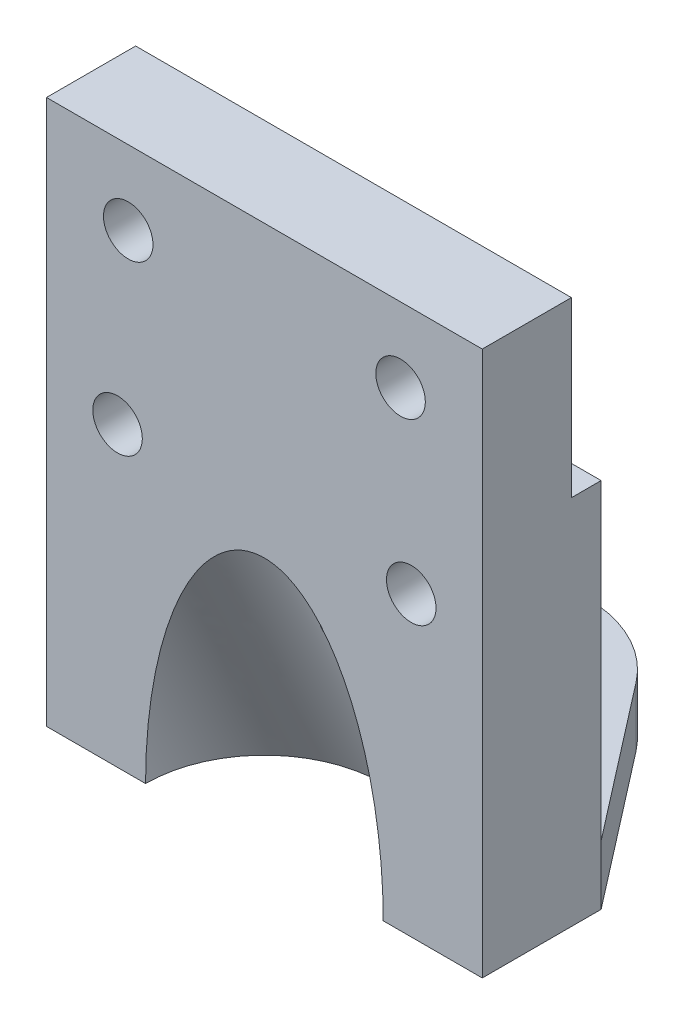
ISO-10303-21;
HEADER;
FILE_DESCRIPTION(('STEP AP214'),'2;1');
FILE_NAME('part.step','',(''),(''),'','','');
FILE_SCHEMA(('AUTOMOTIVE_DESIGN { 1 0 10303 214 1 1 1 1 }'));
ENDSEC;
DATA;
#1=APPLICATION_CONTEXT('core data for automotive mechanical design processes');
#2=APPLICATION_PROTOCOL_DEFINITION('international standard','automotive_design',2000,#1);
#3=PRODUCT_CONTEXT('',#1,'mechanical');
#4=PRODUCT('Part','Part','',(#3));
#5=PRODUCT_RELATED_PRODUCT_CATEGORY('part','',(#4));
#6=PRODUCT_DEFINITION_FORMATION('','',#4);
#7=PRODUCT_DEFINITION_CONTEXT('part definition',#1,'design');
#8=PRODUCT_DEFINITION('design','',#6,#7);
#9=PRODUCT_DEFINITION_SHAPE('','',#8);
#10=(LENGTH_UNIT() NAMED_UNIT(*) SI_UNIT(.MILLI.,.METRE.));
#11=(NAMED_UNIT(*) PLANE_ANGLE_UNIT() SI_UNIT($,.RADIAN.));
#12=(NAMED_UNIT(*) SI_UNIT($,.STERADIAN.) SOLID_ANGLE_UNIT());
#13=UNCERTAINTY_MEASURE_WITH_UNIT(LENGTH_MEASURE(1.E-05),#10,'distance_accuracy_value','');
#14=(GEOMETRIC_REPRESENTATION_CONTEXT(3) GLOBAL_UNCERTAINTY_ASSIGNED_CONTEXT((#13)) GLOBAL_UNIT_ASSIGNED_CONTEXT((#10,
#11,#12)) REPRESENTATION_CONTEXT('',''));
#15=CARTESIAN_POINT('',(0.,0.,0.));
#16=DIRECTION('',(0.,0.,1.));
#17=DIRECTION('',(1.,0.,0.));
#18=AXIS2_PLACEMENT_3D('',#15,#16,#17);
#19=CARTESIAN_POINT('',(-44.,75.,-24.));
#20=DIRECTION('',(0.,0.,1.));
#21=DIRECTION('',(1.,0.,0.));
#22=AXIS2_PLACEMENT_3D('',#19,#20,#21);
#23=PLANE('',#22);
#24=CARTESIAN_POINT('',(-29.6529204550313,60.,-24.));
#25=DIRECTION('',(0.,0.,1.));
#26=DIRECTION('',(1.,0.,0.));
#27=AXIS2_PLACEMENT_3D('',#24,#25,#26);
#28=CIRCLE('',#27,5.);
#29=CARTESIAN_POINT('',(-24.6529204550313,60.,-24.));
#30=VERTEX_POINT('',#29);
#31=EDGE_CURVE('E140',#30,#30,#28,.F.);
#32=ORIENTED_EDGE('',*,*,#31,.F.);
#33=EDGE_LOOP('',(#32));
#34=FACE_BOUND('',#33,.T.);
#35=CARTESIAN_POINT('',(29.6529204550313,60.,-24.));
#36=DIRECTION('',(0.,0.,1.));
#37=DIRECTION('',(1.,0.,0.));
#38=AXIS2_PLACEMENT_3D('',#35,#36,#37);
#39=CIRCLE('',#38,5.);
#40=CARTESIAN_POINT('',(34.6529204550313,60.,-24.));
#41=VERTEX_POINT('',#40);
#42=EDGE_CURVE('E257',#41,#41,#39,.F.);
#43=ORIENTED_EDGE('',*,*,#42,.F.);
#44=EDGE_LOOP('',(#43));
#45=FACE_BOUND('',#44,.T.);
#46=DIRECTION('',(1.,0.,0.));
#47=VECTOR('',#46,1.);
#48=CARTESIAN_POINT('',(0.,12.,-24.));
#49=LINE('',#48,#47);
#50=CARTESIAN_POINT('',(-44.,12.,-24.));
#51=VERTEX_POINT('',#50);
#52=CARTESIAN_POINT('',(44.,12.,-24.));
#53=VERTEX_POINT('',#52);
#54=EDGE_CURVE('E75',#51,#53,#49,.T.);
#55=ORIENTED_EDGE('',*,*,#54,.F.);
#56=DIRECTION('',(0.,-1.,0.));
#57=VECTOR('',#56,1.);
#58=CARTESIAN_POINT('',(-44.,75.,-24.));
#59=LINE('',#58,#57);
#60=CARTESIAN_POINT('',(-44.,75.,-24.));
#61=VERTEX_POINT('',#60);
#62=EDGE_CURVE('E221',#61,#51,#59,.T.);
#63=ORIENTED_EDGE('',*,*,#62,.F.);
#64=DIRECTION('',(-1.,0.,0.));
#65=VECTOR('',#64,1.);
#66=CARTESIAN_POINT('',(-44.,75.,-24.));
#67=LINE('',#66,#65);
#68=CARTESIAN_POINT('',(44.,75.,-24.));
#69=VERTEX_POINT('',#68);
#70=EDGE_CURVE('E211',#69,#61,#67,.T.);
#71=ORIENTED_EDGE('',*,*,#70,.F.);
#72=DIRECTION('',(0.,-1.,0.));
#73=VECTOR('',#72,1.);
#74=CARTESIAN_POINT('',(44.,75.,-24.));
#75=LINE('',#74,#73);
#76=EDGE_CURVE('E172',#69,#53,#75,.T.);
#77=ORIENTED_EDGE('',*,*,#76,.T.);
#78=EDGE_LOOP('',(#55,#63,#71,#77));
#79=FACE_BOUND('',#78,.T.);
#80=ADVANCED_FACE('F44',(#34,#45,#79),#23,.F.);
#81=CARTESIAN_POINT('',(0.,0.,-18.));
#82=DIRECTION('',(0.,0.,1.));
#83=DIRECTION('',(1.,0.,0.));
#84=AXIS2_PLACEMENT_3D('',#81,#82,#83);
#85=PLANE('',#84);
#86=CARTESIAN_POINT('',(27.5,95.,-18.));
#87=DIRECTION('',(0.,0.,1.));
#88=DIRECTION('',(1.,0.,0.));
#89=AXIS2_PLACEMENT_3D('',#86,#87,#88);
#90=CIRCLE('',#89,5.);
#91=CARTESIAN_POINT('',(32.5,95.,-18.));
#92=VERTEX_POINT('',#91);
#93=EDGE_CURVE('E199',#92,#92,#90,.T.);
#94=ORIENTED_EDGE('',*,*,#93,.T.);
#95=EDGE_LOOP('',(#94));
#96=FACE_BOUND('',#95,.T.);
#97=CARTESIAN_POINT('',(-27.5,95.,-18.));
#98=DIRECTION('',(0.,0.,1.));
#99=DIRECTION('',(1.,0.,0.));
#100=AXIS2_PLACEMENT_3D('',#97,#98,#99);
#101=CIRCLE('',#100,5.);
#102=CARTESIAN_POINT('',(-22.5,95.,-18.));
#103=VERTEX_POINT('',#102);
#104=EDGE_CURVE('E246',#103,#103,#101,.T.);
#105=ORIENTED_EDGE('',*,*,#104,.T.);
#106=EDGE_LOOP('',(#105));
#107=FACE_BOUND('',#106,.T.);
#108=DIRECTION('',(1.,0.,0.));
#109=VECTOR('',#108,1.);
#110=CARTESIAN_POINT('',(-44.,75.,-18.));
#111=LINE('',#110,#109);
#112=CARTESIAN_POINT('',(-44.,75.,-18.));
#113=VERTEX_POINT('',#112);
#114=CARTESIAN_POINT('',(44.,75.,-18.));
#115=VERTEX_POINT('',#114);
#116=EDGE_CURVE('E220',#113,#115,#111,.T.);
#117=ORIENTED_EDGE('',*,*,#116,.F.);
#118=DIRECTION('',(0.,-1.,0.));
#119=VECTOR('',#118,1.);
#120=CARTESIAN_POINT('',(-44.,110.,-18.));
#121=LINE('',#120,#119);
#122=CARTESIAN_POINT('',(-44.,110.,-18.));
#123=VERTEX_POINT('',#122);
#124=EDGE_CURVE('E160',#123,#113,#121,.T.);
#125=ORIENTED_EDGE('',*,*,#124,.F.);
#126=DIRECTION('',(-1.,0.,0.));
#127=VECTOR('',#126,1.);
#128=CARTESIAN_POINT('',(-44.,110.,-18.));
#129=LINE('',#128,#127);
#130=CARTESIAN_POINT('',(44.,110.,-18.));
#131=VERTEX_POINT('',#130);
#132=EDGE_CURVE('E150',#131,#123,#129,.T.);
#133=ORIENTED_EDGE('',*,*,#132,.F.);
#134=DIRECTION('',(0.,1.,0.));
#135=VECTOR('',#134,1.);
#136=CARTESIAN_POINT('',(44.,110.,-18.));
#137=LINE('',#136,#135);
#138=EDGE_CURVE('E143',#115,#131,#137,.T.);
#139=ORIENTED_EDGE('',*,*,#138,.F.);
#140=EDGE_LOOP('',(#117,#125,#133,#139));
#141=FACE_BOUND('',#140,.T.);
#142=ADVANCED_FACE('F310',(#96,#107,#141),#85,.F.);
#143=CARTESIAN_POINT('',(44.,110.,-18.));
#144=DIRECTION('',(1.,0.,0.));
#145=DIRECTION('',(0.,1.,0.));
#146=AXIS2_PLACEMENT_3D('',#143,#144,#145);
#147=PLANE('',#146);
#148=DIRECTION('',(0.,1.,0.));
#149=VECTOR('',#148,1.);
#150=CARTESIAN_POINT('',(44.,110.,0.));
#151=LINE('',#150,#149);
#152=CARTESIAN_POINT('',(44.,0.,0.));
#153=VERTEX_POINT('',#152);
#154=CARTESIAN_POINT('',(44.,110.,0.));
#155=VERTEX_POINT('',#154);
#156=EDGE_CURVE('E171',#153,#155,#151,.T.);
#157=ORIENTED_EDGE('',*,*,#156,.F.);
#158=DIRECTION('',(0.,0.,1.));
#159=VECTOR('',#158,1.);
#160=CARTESIAN_POINT('',(44.,0.,-18.));
#161=LINE('',#160,#159);
#162=CARTESIAN_POINT('',(44.,0.,-24.));
#163=VERTEX_POINT('',#162);
#164=EDGE_CURVE('E56',#163,#153,#161,.T.);
#165=ORIENTED_EDGE('',*,*,#164,.F.);
#166=DIRECTION('',(0.,-1.,0.));
#167=VECTOR('',#166,1.);
#168=CARTESIAN_POINT('',(44.,12.,-24.));
#169=LINE('',#168,#167);
#170=EDGE_CURVE('E207',#53,#163,#169,.T.);
#171=ORIENTED_EDGE('',*,*,#170,.F.);
#172=ORIENTED_EDGE('',*,*,#76,.F.);
#173=DIRECTION('',(0.,0.,-1.));
#174=VECTOR('',#173,1.);
#175=CARTESIAN_POINT('',(44.,75.,-24.));
#176=LINE('',#175,#174);
#177=EDGE_CURVE('E204',#115,#69,#176,.T.);
#178=ORIENTED_EDGE('',*,*,#177,.F.);
#179=ORIENTED_EDGE('',*,*,#138,.T.);
#180=DIRECTION('',(0.,0.,1.));
#181=VECTOR('',#180,1.);
#182=CARTESIAN_POINT('',(44.,110.,-18.));
#183=LINE('',#182,#181);
#184=EDGE_CURVE('E156',#131,#155,#183,.T.);
#185=ORIENTED_EDGE('',*,*,#184,.T.);
#186=EDGE_LOOP('',(#157,#165,#171,#172,#178,#179,#185));
#187=FACE_BOUND('',#186,.T.);
#188=ADVANCED_FACE('F50',(#187),#147,.T.);
#189=CARTESIAN_POINT('',(-44.,0.,-18.));
#190=DIRECTION('',(0.,-1.,0.));
#191=DIRECTION('',(0.,0.,-1.));
#192=AXIS2_PLACEMENT_3D('',#189,#190,#191);
#193=PLANE('',#192);
#194=CARTESIAN_POINT('',(0.,0.,0.));
#195=DIRECTION('',(0.,-1.,0.));
#196=DIRECTION('',(0.,0.,-1.));
#197=AXIS2_PLACEMENT_3D('',#194,#195,#196);
#198=CIRCLE('',#197,24.);
#199=CARTESIAN_POINT('',(-24.,0.,0.));
#200=VERTEX_POINT('',#199);
#201=CARTESIAN_POINT('',(24.,0.,0.));
#202=VERTEX_POINT('',#201);
#203=EDGE_CURVE('E61',#200,#202,#198,.T.);
#204=ORIENTED_EDGE('',*,*,#203,.F.);
#205=DIRECTION('',(1.,0.,0.));
#206=VECTOR('',#205,1.);
#207=CARTESIAN_POINT('',(-44.,0.,0.));
#208=LINE('',#207,#206);
#209=CARTESIAN_POINT('',(-44.,0.,0.));
#210=VERTEX_POINT('',#209);
#211=EDGE_CURVE('E131',#210,#200,#208,.T.);
#212=ORIENTED_EDGE('',*,*,#211,.F.);
#213=DIRECTION('',(0.,0.,1.));
#214=VECTOR('',#213,1.);
#215=CARTESIAN_POINT('',(-44.,0.,-18.));
#216=LINE('',#215,#214);
#217=CARTESIAN_POINT('',(-44.,0.,-24.));
#218=VERTEX_POINT('',#217);
#219=EDGE_CURVE('E155',#218,#210,#216,.T.);
#220=ORIENTED_EDGE('',*,*,#219,.F.);
#221=DIRECTION('',(0.612114706356877,0.,-0.790768984129773));
#222=VECTOR('',#221,1.);
#223=CARTESIAN_POINT('',(-39.1308775839132,0.,-30.2902442084566));
#224=LINE('',#223,#222);
#225=CARTESIAN_POINT('',(-19.7692246032443,0.,-55.3028676589219));
#226=VERTEX_POINT('',#225);
#227=EDGE_CURVE('E183',#218,#226,#224,.T.);
#228=ORIENTED_EDGE('',*,*,#227,.T.);
#229=CARTESIAN_POINT('',(0.,0.,-40.));
#230=DIRECTION('',(0.,-1.,0.));
#231=DIRECTION('',(0.,0.,-1.));
#232=AXIS2_PLACEMENT_3D('',#229,#230,#231);
#233=CIRCLE('',#232,25.);
#234=CARTESIAN_POINT('',(19.7692246032443,0.,-55.3028676589219));
#235=VERTEX_POINT('',#234);
#236=EDGE_CURVE('E192',#226,#235,#233,.T.);
#237=ORIENTED_EDGE('',*,*,#236,.T.);
#238=DIRECTION('',(0.612114706356877,0.,0.790768984129774));
#239=VECTOR('',#238,1.);
#240=CARTESIAN_POINT('',(39.1308775839132,0.,-30.2902442084566));
#241=LINE('',#240,#239);
#242=EDGE_CURVE('E191',#235,#163,#241,.T.);
#243=ORIENTED_EDGE('',*,*,#242,.T.);
#244=ORIENTED_EDGE('',*,*,#164,.T.);
#245=EDGE_CURVE('E136',#202,#153,#208,.T.);
#246=ORIENTED_EDGE('',*,*,#245,.F.);
#247=EDGE_LOOP('',(#204,#212,#220,#228,#237,#243,#244,#246));
#248=FACE_BOUND('',#247,.T.);
#249=CARTESIAN_POINT('',(0.,0.,-40.));
#250=DIRECTION('',(0.,-1.,0.));
#251=DIRECTION('',(0.,0.,-1.));
#252=AXIS2_PLACEMENT_3D('',#249,#250,#251);
#253=CIRCLE('',#252,9.5);
#254=CARTESIAN_POINT('',(0.,0.,-49.5));
#255=VERTEX_POINT('',#254);
#256=EDGE_CURVE('E195',#255,#255,#253,.T.);
#257=ORIENTED_EDGE('',*,*,#256,.F.);
#258=EDGE_LOOP('',(#257));
#259=FACE_BOUND('',#258,.T.);
#260=ADVANCED_FACE('F132',(#248,#259),#193,.T.);
#261=CARTESIAN_POINT('',(-44.,110.,-18.));
#262=DIRECTION('',(-1.,0.,0.));
#263=DIRECTION('',(0.,-1.,0.));
#264=AXIS2_PLACEMENT_3D('',#261,#262,#263);
#265=PLANE('',#264);
#266=DIRECTION('',(0.,-1.,0.));
#267=VECTOR('',#266,1.);
#268=CARTESIAN_POINT('',(-44.,110.,0.));
#269=LINE('',#268,#267);
#270=CARTESIAN_POINT('',(-44.,110.,0.));
#271=VERTEX_POINT('',#270);
#272=EDGE_CURVE('E144',#271,#210,#269,.T.);
#273=ORIENTED_EDGE('',*,*,#272,.F.);
#274=DIRECTION('',(0.,0.,1.));
#275=VECTOR('',#274,1.);
#276=CARTESIAN_POINT('',(-44.,110.,-18.));
#277=LINE('',#276,#275);
#278=EDGE_CURVE('E153',#123,#271,#277,.T.);
#279=ORIENTED_EDGE('',*,*,#278,.F.);
#280=ORIENTED_EDGE('',*,*,#124,.T.);
#281=DIRECTION('',(0.,0.,1.));
#282=VECTOR('',#281,1.);
#283=CARTESIAN_POINT('',(-44.,75.,-24.));
#284=LINE('',#283,#282);
#285=EDGE_CURVE('E217',#61,#113,#284,.T.);
#286=ORIENTED_EDGE('',*,*,#285,.F.);
#287=ORIENTED_EDGE('',*,*,#62,.T.);
#288=DIRECTION('',(0.,-1.,0.));
#289=VECTOR('',#288,1.);
#290=CARTESIAN_POINT('',(-44.,12.,-24.));
#291=LINE('',#290,#289);
#292=EDGE_CURVE('E179',#51,#218,#291,.T.);
#293=ORIENTED_EDGE('',*,*,#292,.T.);
#294=ORIENTED_EDGE('',*,*,#219,.T.);
#295=EDGE_LOOP('',(#273,#279,#280,#286,#287,#293,#294));
#296=FACE_BOUND('',#295,.T.);
#297=ADVANCED_FACE('F178',(#296),#265,.T.);
#298=CARTESIAN_POINT('',(-44.,110.,-18.));
#299=DIRECTION('',(0.,1.,0.));
#300=DIRECTION('',(0.,0.,1.));
#301=AXIS2_PLACEMENT_3D('',#298,#299,#300);
#302=PLANE('',#301);
#303=DIRECTION('',(-1.,0.,0.));
#304=VECTOR('',#303,1.);
#305=CARTESIAN_POINT('',(-44.,110.,0.));
#306=LINE('',#305,#304);
#307=EDGE_CURVE('E173',#155,#271,#306,.T.);
#308=ORIENTED_EDGE('',*,*,#307,.F.);
#309=ORIENTED_EDGE('',*,*,#184,.F.);
#310=ORIENTED_EDGE('',*,*,#132,.T.);
#311=ORIENTED_EDGE('',*,*,#278,.T.);
#312=EDGE_LOOP('',(#308,#309,#310,#311));
#313=FACE_BOUND('',#312,.T.);
#314=ADVANCED_FACE('F176',(#313),#302,.T.);
#315=CARTESIAN_POINT('',(0.,0.,0.));
#316=DIRECTION('',(0.,0.,1.));
#317=DIRECTION('',(1.,0.,0.));
#318=AXIS2_PLACEMENT_3D('',#315,#316,#317);
#319=PLANE('',#318);
#320=CARTESIAN_POINT('',(24.,0.,0.));
#321=CARTESIAN_POINT('',(23.9999836526665,0.822487909594253,0.));
#322=CARTESIAN_POINT('',(23.9908057653102,1.64497853466898,0.));
#323=CARTESIAN_POINT('',(23.9540097607918,3.28956132881042,0.));
#324=CARTESIAN_POINT('',(23.926391316428,4.11165349054796,0.));
#325=CARTESIAN_POINT('',(23.8525962581262,5.75502367391495,0.));
#326=CARTESIAN_POINT('',(23.8064192507315,6.57630167791351,0.));
#327=CARTESIAN_POINT('',(23.6952719286014,8.21758441968101,0.));
#328=CARTESIAN_POINT('',(23.6303016801107,9.03758916192785,0.));
#329=CARTESIAN_POINT('',(23.4812324663408,10.6759416559738,0.));
#330=CARTESIAN_POINT('',(23.3971316451274,11.4942892392287,0.));
#331=CARTESIAN_POINT('',(23.2093684539698,13.1287360620571,0.));
#332=CARTESIAN_POINT('',(23.1057062152105,13.9448353166713,0.));
#333=CARTESIAN_POINT('',(22.8782379124427,15.5744315564589,0.));
#334=CARTESIAN_POINT('',(22.7544269129195,16.3879278541186,0.));
#335=CARTESIAN_POINT('',(22.4859934425246,18.011484999328,0.));
#336=CARTESIAN_POINT('',(22.3413710215974,18.8215458551175,0.));
#337=CARTESIAN_POINT('',(22.0303366920778,20.4382530974152,0.));
#338=CARTESIAN_POINT('',(21.8639049278322,21.2448956725252,0.));
#339=CARTESIAN_POINT('',(21.5083419460309,22.8531858262733,0.));
#340=CARTESIAN_POINT('',(21.3192104530091,23.6548333441712,0.));
#341=CARTESIAN_POINT('',(20.9171806973682,25.2515514932186,0.));
#342=CARTESIAN_POINT('',(20.7042994691011,26.0466264044593,0.));
#343=CARTESIAN_POINT('',(20.2532181884177,27.6295613335899,0.));
#344=CARTESIAN_POINT('',(20.0150191240817,28.4174216317423,0.));
#345=CARTESIAN_POINT('',(19.5811011965835,29.7680075743554,0.));
#346=CARTESIAN_POINT('',(19.3918229003344,30.3328070716185,0.));
#347=CARTESIAN_POINT('',(18.9983197094544,31.4571678498858,0.));
#348=CARTESIAN_POINT('',(18.7940953229582,32.0167293082431,0.));
#349=CARTESIAN_POINT('',(18.3694400982678,33.1308226792633,0.));
#350=CARTESIAN_POINT('',(18.1489810141352,33.6853438457671,0.));
#351=CARTESIAN_POINT('',(17.6911520653764,34.7874175427981,0.));
#352=CARTESIAN_POINT('',(17.4537810886212,35.3349696122406,0.));
#353=CARTESIAN_POINT('',(16.9476076228236,36.4514129876872,0.));
#354=CARTESIAN_POINT('',(16.6777984072819,37.0198493617967,0.));
#355=CARTESIAN_POINT('',(16.1165136512702,38.1460542111866,0.));
#356=CARTESIAN_POINT('',(15.8250350867354,38.7038211837916,0.));
#357=CARTESIAN_POINT('',(15.2185176396709,39.8067451213144,0.));
#358=CARTESIAN_POINT('',(14.9034689307155,40.3518967014499,0.));
#359=CARTESIAN_POINT('',(14.2485810107537,41.4254938166613,0.));
#360=CARTESIAN_POINT('',(13.9087988632846,41.9539740118063,0.));
#361=CARTESIAN_POINT('',(13.2016085396942,42.9919404479344,0.));
#362=CARTESIAN_POINT('',(12.8342094297376,43.5014328408329,0.));
#363=CARTESIAN_POINT('',(12.069337180971,44.4968967678886,0.));
#364=CARTESIAN_POINT('',(11.6718869671355,44.9828857770432,0.));
#365=CARTESIAN_POINT('',(10.9571341392998,45.7970048330569,0.));
#366=CARTESIAN_POINT('',(10.6476189755373,46.1319738134576,0.));
#367=CARTESIAN_POINT('',(10.0100534463654,46.7838605800252,0.));
#368=CARTESIAN_POINT('',(9.68200361255512,47.1007788833865,0.));
#369=CARTESIAN_POINT('',(9.00651320728129,47.7130922602464,0.));
#370=CARTESIAN_POINT('',(8.65907904533572,48.008494374558,0.));
#371=CARTESIAN_POINT('',(7.94400137484032,48.5738150243813,0.));
#372=CARTESIAN_POINT('',(7.5763606976892,48.8437371159008,0.));
#373=CARTESIAN_POINT('',(6.87842333286768,49.3143270688157,0.));
#374=CARTESIAN_POINT('',(6.55101640742542,49.5192727016577,0.));
#375=CARTESIAN_POINT('',(5.88182559725525,49.9041118924472,0.));
#376=CARTESIAN_POINT('',(5.54004565729388,50.0840122665497,0.));
#377=CARTESIAN_POINT('',(4.84325019996284,50.4150771658752,0.));
#378=CARTESIAN_POINT('',(4.48825034666849,50.5662744815447,0.));
#379=CARTESIAN_POINT('',(3.76620929190656,50.8365690620231,0.));
#380=CARTESIAN_POINT('',(3.39917058928302,50.9556729415999,0.));
#381=CARTESIAN_POINT('',(2.71720419195341,51.1416375447859,0.));
#382=CARTESIAN_POINT('',(2.40374299216621,51.2138891160395,0.));
#383=CARTESIAN_POINT('',(1.77191133618509,51.3322053022059,0.));
#384=CARTESIAN_POINT('',(1.45354140996074,51.3782727240299,0.));
#385=CARTESIAN_POINT('',(0.814160316802971,51.4431196132183,0.));
#386=CARTESIAN_POINT('',(0.493150343335911,51.4619107952871,0.));
#387=CARTESIAN_POINT('',(-0.149306775880375,51.4717802967483,0.));
#388=CARTESIAN_POINT('',(-0.470753932361496,51.4628579230955,0.));
#389=CARTESIAN_POINT('',(-1.1114281321947,51.4175388112742,0.));
#390=CARTESIAN_POINT('',(-1.43065678546214,51.3811646984799,0.));
#391=CARTESIAN_POINT('',(-2.06492350818319,51.2818472771285,0.));
#392=CARTESIAN_POINT('',(-2.37996164925039,51.2189044232202,0.));
#393=CARTESIAN_POINT('',(-3.00410626600889,51.0678220922029,0.));
#394=CARTESIAN_POINT('',(-3.31320912765997,50.9796677522938,0.));
#395=CARTESIAN_POINT('',(-3.92375753208044,50.7799834702479,0.));
#396=CARTESIAN_POINT('',(-4.22520204538625,50.6684504039024,0.));
#397=CARTESIAN_POINT('',(-4.92735187034173,50.3795418980444,0.));
#398=CARTESIAN_POINT('',(-5.32428867972908,50.1929723214894,0.));
#399=CARTESIAN_POINT('',(-6.10001899917514,49.7853385604929,0.));
#400=CARTESIAN_POINT('',(-6.47880602172513,49.5642621602939,0.));
#401=CARTESIAN_POINT('',(-7.21818902793007,49.0922008508507,0.));
#402=CARTESIAN_POINT('',(-7.57874828598963,48.8411587372866,0.));
#403=CARTESIAN_POINT('',(-8.28093653709508,48.3140083696173,0.));
#404=CARTESIAN_POINT('',(-8.62256542370406,48.0378999745988,0.));
#405=CARTESIAN_POINT('',(-9.31547347394543,47.4402993485481,0.));
#406=CARTESIAN_POINT('',(-9.66513951450063,47.1169433940486,0.));
#407=CARTESIAN_POINT('',(-10.3440792845559,46.4492271115206,0.));
#408=CARTESIAN_POINT('',(-10.6733414076691,46.1048550459444,0.));
#409=CARTESIAN_POINT('',(-11.3125422271333,45.3985418051512,0.));
#410=CARTESIAN_POINT('',(-11.6224763711099,45.0365965263012,0.));
#411=CARTESIAN_POINT('',(-12.2246309056722,44.2973811776463,0.));
#412=CARTESIAN_POINT('',(-12.5168231800207,43.9200882884172,0.));
#413=CARTESIAN_POINT('',(-13.0840826830311,43.1530623864951,0.));
#414=CARTESIAN_POINT('',(-13.3591553212788,42.7633333629512,0.));
#415=CARTESIAN_POINT('',(-13.8933730547424,41.9731799243,0.));
#416=CARTESIAN_POINT('',(-14.15251908523,41.5727561392151,0.));
#417=CARTESIAN_POINT('',(-14.7680045471288,40.5823778895924,0.));
#418=CARTESIAN_POINT('',(-15.116263206689,39.9873942509957,0.));
#419=CARTESIAN_POINT('',(-15.7844863843685,38.7818271839245,0.));
#420=CARTESIAN_POINT('',(-16.1044503091856,38.1712434286825,0.));
#421=CARTESIAN_POINT('',(-16.7180480719262,36.9380595468113,0.));
#422=CARTESIAN_POINT('',(-17.0117170838991,36.3154768686512,0.));
#423=CARTESIAN_POINT('',(-17.5752287733984,35.0596665326451,0.));
#424=CARTESIAN_POINT('',(-17.8450717647895,34.4264390151565,0.));
#425=CARTESIAN_POINT('',(-18.3620936655649,33.1524549565529,0.));
#426=CARTESIAN_POINT('',(-18.6093214058529,32.5117181767814,0.));
#427=CARTESIAN_POINT('',(-19.0832530838873,31.2227182470839,0.));
#428=CARTESIAN_POINT('',(-19.309957031408,30.5744551007426,0.));
#429=CARTESIAN_POINT('',(-19.7441491953644,29.2713826814665,0.));
#430=CARTESIAN_POINT('',(-19.9516332097714,28.6165720115627,0.));
#431=CARTESIAN_POINT('',(-20.3484119651296,27.3014761201153,0.));
#432=CARTESIAN_POINT('',(-20.5377067285607,26.6411909053388,0.));
#433=CARTESIAN_POINT('',(-20.8988504344434,25.3166196544326,0.));
#434=CARTESIAN_POINT('',(-21.0707175405811,24.6523385642874,0.));
#435=CARTESIAN_POINT('',(-21.3980301208407,23.3197334732271,0.));
#436=CARTESIAN_POINT('',(-21.5534749308115,22.6514093099567,0.));
#437=CARTESIAN_POINT('',(-21.9961869663252,20.6414343273693,0.));
#438=CARTESIAN_POINT('',(-22.2598972755839,19.2945384759662,0.));
#439=CARTESIAN_POINT('',(-22.7501360871939,16.4680069186354,0.));
#440=CARTESIAN_POINT('',(-22.9711171706571,14.9874193121596,0.));
#441=CARTESIAN_POINT('',(-23.3475935080462,12.0177936868394,0.));
#442=CARTESIAN_POINT('',(-23.5030824528849,10.528754867857,0.));
#443=CARTESIAN_POINT('',(-23.6896257618222,8.28573125678749,0.));
#444=CARTESIAN_POINT('',(-23.7441417521579,7.53361535749895,0.));
#445=CARTESIAN_POINT('',(-23.8374320196193,6.02839246019668,0.));
#446=CARTESIAN_POINT('',(-23.8762062439604,5.27528545886812,0.));
#447=CARTESIAN_POINT('',(-23.93817239567,3.76863577622158,0.));
#448=CARTESIAN_POINT('',(-23.9613684588128,3.01509326373893,0.));
#449=CARTESIAN_POINT('',(-23.9922764764292,1.50770052084697,0.));
#450=CARTESIAN_POINT('',(-23.9999886377953,0.753850294683881,0.));
#451=CARTESIAN_POINT('',(-24.,0.,0.));
#452=B_SPLINE_CURVE_WITH_KNOTS('',3,(#320,#321,#322,#323,#324,#325,#326,#327,#328,#329,#330,
#331,#332,#333,#334,#335,#336,#337,#338,#339,#340,#341,#342,#343,#344,#345,#346,#347,#348,#349,
#350,#351,#352,#353,#354,#355,#356,#357,#358,#359,#360,#361,#362,#363,#364,#365,#366,#367,#368,
#369,#370,#371,#372,#373,#374,#375,#376,#377,#378,#379,#380,#381,#382,#383,#384,#385,#386,#387,
#388,#389,#390,#391,#392,#393,#394,#395,#396,#397,#398,#399,#400,#401,#402,#403,#404,#405,#406,
#407,#408,#409,#410,#411,#412,#413,#414,#415,#416,#417,#418,#419,#420,#421,#422,#423,#424,#425,
#426,#427,#428,#429,#430,#431,#432,#433,#434,#435,#436,#437,#438,#439,#440,#441,#442,#443,#444,
#445,#446,#447,#448,#449,#450,#451),.UNSPECIFIED.,.F.,.F.,(4,2,2,2,2,2,2,2,2,2,2,2,2,2,2,2,2,2,
2,2,2,2,2,2,2,2,2,2,2,2,2,2,2,2,2,2,2,2,2,2,2,2,2,2,2,2,2,2,2,2,2,2,2,2,2,2,2,2,2,2,2,2,2,2,2,
4),(0.,2.46741691644283,4.93487761489322,7.40239062828775,9.86989494399663,12.3376387444532,
14.8053659960386,17.2736986390724,19.7420253585442,22.2126151098192,24.6832348452831,
27.1520938001287,29.6208564380626,31.4076847790444,33.1944523999212,34.9844057215462,
36.7744768596513,38.6617113170035,40.5492096434444,42.4374993032028,44.3215626516591,
46.2050101738528,48.0870350993933,49.4546328272379,50.8221913504468,52.1893003335402,
53.5562182391101,54.7140469673573,55.8715599698664,57.027742562412,58.1836866719385,
59.1476976008054,60.1116051692906,61.075098632429,62.0386161902714,63.0013404952501,
63.9640483265969,64.9273248722699,65.8907302272614,67.2044881409366,68.5187121972032,
69.8354864749469,71.1522681555657,72.5800231963346,74.0085830716977,75.4374781588577,
76.86858155224,78.2992304149496,79.7297951840103,81.7971160690803,83.8644802927963,
85.9290363978916,87.9935653021304,90.0535257105647,92.1134851379491,94.1738938738373,
96.2343000632634,98.2925362668623,100.350855677872,104.466741611147,108.956210356089,
113.446111488422,115.708245553519,117.97038720384,120.23192805092,122.493438679569),.UNSPECIFIED.);
#453=EDGE_CURVE('E11',#202,#200,#452,.T.);
#454=ORIENTED_EDGE('',*,*,#453,.F.);
#455=ORIENTED_EDGE('',*,*,#245,.T.);
#456=ORIENTED_EDGE('',*,*,#156,.T.);
#457=ORIENTED_EDGE('',*,*,#307,.T.);
#458=ORIENTED_EDGE('',*,*,#272,.T.);
#459=ORIENTED_EDGE('',*,*,#211,.T.);
#460=EDGE_LOOP('',(#454,#455,#456,#457,#458,#459));
#461=FACE_BOUND('',#460,.T.);
#462=CARTESIAN_POINT('',(-29.6529204550313,60.,0.));
#463=DIRECTION('',(0.,0.,1.));
#464=DIRECTION('',(1.,0.,0.));
#465=AXIS2_PLACEMENT_3D('',#462,#463,#464);
#466=CIRCLE('',#465,5.);
#467=CARTESIAN_POINT('',(-24.6529204550313,60.,0.));
#468=VERTEX_POINT('',#467);
#469=EDGE_CURVE('E254',#468,#468,#466,.T.);
#470=ORIENTED_EDGE('',*,*,#469,.F.);
#471=EDGE_LOOP('',(#470));
#472=FACE_BOUND('',#471,.T.);
#473=CARTESIAN_POINT('',(29.6529204550313,60.,0.));
#474=DIRECTION('',(0.,0.,1.));
#475=DIRECTION('',(1.,0.,0.));
#476=AXIS2_PLACEMENT_3D('',#473,#474,#475);
#477=CIRCLE('',#476,5.);
#478=CARTESIAN_POINT('',(34.6529204550313,60.,0.));
#479=VERTEX_POINT('',#478);
#480=EDGE_CURVE('E256',#479,#479,#477,.T.);
#481=ORIENTED_EDGE('',*,*,#480,.F.);
#482=EDGE_LOOP('',(#481));
#483=FACE_BOUND('',#482,.T.);
#484=CARTESIAN_POINT('',(27.5,95.,0.));
#485=DIRECTION('',(0.,0.,1.));
#486=DIRECTION('',(1.,0.,0.));
#487=AXIS2_PLACEMENT_3D('',#484,#485,#486);
#488=CIRCLE('',#487,5.);
#489=CARTESIAN_POINT('',(32.5,95.,0.));
#490=VERTEX_POINT('',#489);
#491=EDGE_CURVE('E255',#490,#490,#488,.T.);
#492=ORIENTED_EDGE('',*,*,#491,.F.);
#493=EDGE_LOOP('',(#492));
#494=FACE_BOUND('',#493,.T.);
#495=CARTESIAN_POINT('',(-27.5,95.,0.));
#496=DIRECTION('',(0.,0.,1.));
#497=DIRECTION('',(1.,0.,0.));
#498=AXIS2_PLACEMENT_3D('',#495,#496,#497);
#499=CIRCLE('',#498,5.);
#500=CARTESIAN_POINT('',(-22.5,95.,0.));
#501=VERTEX_POINT('',#500);
#502=EDGE_CURVE('E248',#501,#501,#499,.T.);
#503=ORIENTED_EDGE('',*,*,#502,.F.);
#504=EDGE_LOOP('',(#503));
#505=FACE_BOUND('',#504,.T.);
#506=ADVANCED_FACE('F139',(#461,#472,#483,#494,#505),#319,.T.);
#507=CARTESIAN_POINT('',(0.,75.,0.));
#508=DIRECTION('',(0.,1.,0.));
#509=DIRECTION('',(0.,0.,1.));
#510=AXIS2_PLACEMENT_3D('',#507,#508,#509);
#511=PLANE('',#510);
#512=ORIENTED_EDGE('',*,*,#177,.T.);
#513=ORIENTED_EDGE('',*,*,#70,.T.);
#514=ORIENTED_EDGE('',*,*,#285,.T.);
#515=ORIENTED_EDGE('',*,*,#116,.T.);
#516=EDGE_LOOP('',(#512,#513,#514,#515));
#517=FACE_BOUND('',#516,.T.);
#518=ADVANCED_FACE('F296',(#517),#511,.T.);
#519=CARTESIAN_POINT('',(-39.1308775839132,12.,-30.2902442084566));
#520=DIRECTION('',(-0.790768984129773,0.,-0.612114706356877));
#521=DIRECTION('',(-0.612114706356877,0.,0.790768984129773));
#522=AXIS2_PLACEMENT_3D('',#519,#520,#521);
#523=PLANE('',#522);
#524=ORIENTED_EDGE('',*,*,#227,.F.);
#525=ORIENTED_EDGE('',*,*,#292,.F.);
#526=DIRECTION('',(0.612114706356877,0.,-0.790768984129773));
#527=VECTOR('',#526,1.);
#528=CARTESIAN_POINT('',(-39.1308775839132,12.,-30.2902442084566));
#529=LINE('',#528,#527);
#530=CARTESIAN_POINT('',(-19.7692246032443,12.,-55.3028676589219));
#531=VERTEX_POINT('',#530);
#532=EDGE_CURVE('E232',#51,#531,#529,.T.);
#533=ORIENTED_EDGE('',*,*,#532,.T.);
#534=DIRECTION('',(0.,-1.,0.));
#535=VECTOR('',#534,1.);
#536=CARTESIAN_POINT('',(-19.7692246032443,12.,-55.3028676589219));
#537=LINE('',#536,#535);
#538=EDGE_CURVE('E186',#531,#226,#537,.T.);
#539=ORIENTED_EDGE('',*,*,#538,.T.);
#540=EDGE_LOOP('',(#524,#525,#533,#539));
#541=FACE_BOUND('',#540,.T.);
#542=ADVANCED_FACE('F187',(#541),#523,.T.);
#543=CARTESIAN_POINT('',(39.1308775839132,12.,-30.2902442084566));
#544=DIRECTION('',(0.790768984129774,0.,-0.612114706356877));
#545=DIRECTION('',(-0.612114706356877,0.,-0.790768984129774));
#546=AXIS2_PLACEMENT_3D('',#543,#544,#545);
#547=PLANE('',#546);
#548=ORIENTED_EDGE('',*,*,#242,.F.);
#549=DIRECTION('',(0.,-1.,0.));
#550=VECTOR('',#549,1.);
#551=CARTESIAN_POINT('',(19.7692246032443,12.,-55.3028676589219));
#552=LINE('',#551,#550);
#553=CARTESIAN_POINT('',(19.7692246032443,12.,-55.3028676589219));
#554=VERTEX_POINT('',#553);
#555=EDGE_CURVE('E209',#554,#235,#552,.T.);
#556=ORIENTED_EDGE('',*,*,#555,.F.);
#557=DIRECTION('',(0.612114706356877,0.,0.790768984129774));
#558=VECTOR('',#557,1.);
#559=CARTESIAN_POINT('',(39.1308775839132,12.,-30.2902442084566));
#560=LINE('',#559,#558);
#561=EDGE_CURVE('E231',#554,#53,#560,.T.);
#562=ORIENTED_EDGE('',*,*,#561,.T.);
#563=ORIENTED_EDGE('',*,*,#170,.T.);
#564=EDGE_LOOP('',(#548,#556,#562,#563));
#565=FACE_BOUND('',#564,.T.);
#566=ADVANCED_FACE('F236',(#565),#547,.T.);
#567=CARTESIAN_POINT('',(0.,12.,-40.));
#568=DIRECTION('',(0.,-1.,0.));
#569=DIRECTION('',(0.,0.,-1.));
#570=AXIS2_PLACEMENT_3D('',#567,#568,#569);
#571=CYLINDRICAL_SURFACE('',#570,9.5);
#572=CARTESIAN_POINT('',(0.,12.,-40.));
#573=DIRECTION('',(0.,-1.,0.));
#574=DIRECTION('',(0.,0.,-1.));
#575=AXIS2_PLACEMENT_3D('',#572,#573,#574);
#576=CIRCLE('',#575,9.5);
#577=CARTESIAN_POINT('',(0.,12.,-49.5));
#578=VERTEX_POINT('',#577);
#579=EDGE_CURVE('E203',#578,#578,#576,.T.);
#580=ORIENTED_EDGE('',*,*,#579,.F.);
#581=EDGE_LOOP('',(#580));
#582=FACE_BOUND('',#581,.T.);
#583=ORIENTED_EDGE('',*,*,#256,.T.);
#584=EDGE_LOOP('',(#583));
#585=FACE_BOUND('',#584,.T.);
#586=ADVANCED_FACE('F292',(#582,#585),#571,.F.);
#587=CARTESIAN_POINT('',(0.,12.,-40.));
#588=DIRECTION('',(0.,-1.,0.));
#589=DIRECTION('',(0.,0.,-1.));
#590=AXIS2_PLACEMENT_3D('',#587,#588,#589);
#591=CYLINDRICAL_SURFACE('',#590,25.);
#592=ORIENTED_EDGE('',*,*,#236,.F.);
#593=ORIENTED_EDGE('',*,*,#538,.F.);
#594=CARTESIAN_POINT('',(0.,12.,-40.));
#595=DIRECTION('',(0.,-1.,0.));
#596=DIRECTION('',(0.,0.,-1.));
#597=AXIS2_PLACEMENT_3D('',#594,#595,#596);
#598=CIRCLE('',#597,25.);
#599=EDGE_CURVE('E240',#531,#554,#598,.T.);
#600=ORIENTED_EDGE('',*,*,#599,.T.);
#601=ORIENTED_EDGE('',*,*,#555,.T.);
#602=EDGE_LOOP('',(#592,#593,#600,#601));
#603=FACE_BOUND('',#602,.T.);
#604=ADVANCED_FACE('F288',(#603),#591,.T.);
#605=CARTESIAN_POINT('',(0.,12.,0.));
#606=DIRECTION('',(0.,-1.,0.));
#607=DIRECTION('',(0.,0.,-1.));
#608=AXIS2_PLACEMENT_3D('',#605,#606,#607);
#609=PLANE('',#608);
#610=ORIENTED_EDGE('',*,*,#579,.T.);
#611=EDGE_LOOP('',(#610));
#612=FACE_BOUND('',#611,.T.);
#613=ORIENTED_EDGE('',*,*,#532,.F.);
#614=ORIENTED_EDGE('',*,*,#54,.T.);
#615=ORIENTED_EDGE('',*,*,#561,.F.);
#616=ORIENTED_EDGE('',*,*,#599,.F.);
#617=EDGE_LOOP('',(#613,#614,#615,#616));
#618=FACE_BOUND('',#617,.T.);
#619=ADVANCED_FACE('F233',(#612,#618),#609,.F.);
#620=CARTESIAN_POINT('',(-27.5,95.,-38.142135623731));
#621=DIRECTION('',(0.,0.,1.));
#622=DIRECTION('',(1.,0.,0.));
#623=AXIS2_PLACEMENT_3D('',#620,#621,#622);
#624=CYLINDRICAL_SURFACE('',#623,5.);
#625=ORIENTED_EDGE('',*,*,#502,.T.);
#626=EDGE_LOOP('',(#625));
#627=FACE_BOUND('',#626,.T.);
#628=ORIENTED_EDGE('',*,*,#104,.F.);
#629=EDGE_LOOP('',(#628));
#630=FACE_BOUND('',#629,.T.);
#631=ADVANCED_FACE('F273',(#627,#630),#624,.F.);
#632=CARTESIAN_POINT('',(27.5,95.,-38.142135623731));
#633=DIRECTION('',(0.,0.,1.));
#634=DIRECTION('',(1.,0.,0.));
#635=AXIS2_PLACEMENT_3D('',#632,#633,#634);
#636=CYLINDRICAL_SURFACE('',#635,5.);
#637=ORIENTED_EDGE('',*,*,#491,.T.);
#638=EDGE_LOOP('',(#637));
#639=FACE_BOUND('',#638,.T.);
#640=ORIENTED_EDGE('',*,*,#93,.F.);
#641=EDGE_LOOP('',(#640));
#642=FACE_BOUND('',#641,.T.);
#643=ADVANCED_FACE('F272',(#639,#642),#636,.F.);
#644=CARTESIAN_POINT('',(29.6529204550313,60.,-38.142135623731));
#645=DIRECTION('',(0.,0.,1.));
#646=DIRECTION('',(1.,0.,0.));
#647=AXIS2_PLACEMENT_3D('',#644,#645,#646);
#648=CYLINDRICAL_SURFACE('',#647,5.);
#649=ORIENTED_EDGE('',*,*,#42,.T.);
#650=EDGE_LOOP('',(#649));
#651=FACE_BOUND('',#650,.T.);
#652=ORIENTED_EDGE('',*,*,#480,.T.);
#653=EDGE_LOOP('',(#652));
#654=FACE_BOUND('',#653,.T.);
#655=ADVANCED_FACE('F274',(#651,#654),#648,.F.);
#656=CARTESIAN_POINT('',(-29.6529204550313,60.,-38.142135623731));
#657=DIRECTION('',(0.,0.,1.));
#658=DIRECTION('',(1.,0.,0.));
#659=AXIS2_PLACEMENT_3D('',#656,#657,#658);
#660=CYLINDRICAL_SURFACE('',#659,5.);
#661=ORIENTED_EDGE('',*,*,#31,.T.);
#662=EDGE_LOOP('',(#661));
#663=FACE_BOUND('',#662,.T.);
#664=ORIENTED_EDGE('',*,*,#469,.T.);
#665=EDGE_LOOP('',(#664));
#666=FACE_BOUND('',#665,.T.);
#667=ADVANCED_FACE('F269',(#663,#666),#660,.F.);
#668=CARTESIAN_POINT('',(0.,84.9602387292128,39.617609958109));
#669=DIRECTION('',(0.,-1.,0.));
#670=DIRECTION('',(0.,0.,-1.));
#671=AXIS2_PLACEMENT_3D('',#668,#669,#670);
#672=CIRCLE('',#671,24.);
#673=DIRECTION('',(0.,-0.906307787036649,-0.422618261740701));
#674=VECTOR('',#673,1.);
#675=SURFACE_OF_LINEAR_EXTRUSION('',#672,#674);
#676=ORIENTED_EDGE('',*,*,#453,.T.);
#677=ORIENTED_EDGE('',*,*,#203,.T.);
#678=EDGE_LOOP('',(#676,#677));
#679=FACE_BOUND('',#678,.T.);
#680=ADVANCED_FACE('F123',(#679),#675,.F.);
#681=CLOSED_SHELL('',(#80,#142,#188,#260,#297,#314,#506,#518,#542,#566,#586,#604,#619,#631,#643,
#655,#667,#680));
#682=MANIFOLD_SOLID_BREP('B2',#681);
#683=ADVANCED_BREP_SHAPE_REPRESENTATION('',(#18,#682),#14);
#684=SHAPE_DEFINITION_REPRESENTATION(#9,#683);
ENDSEC;
END-ISO-10303-21;
